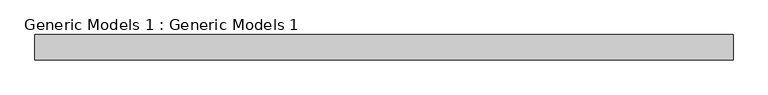
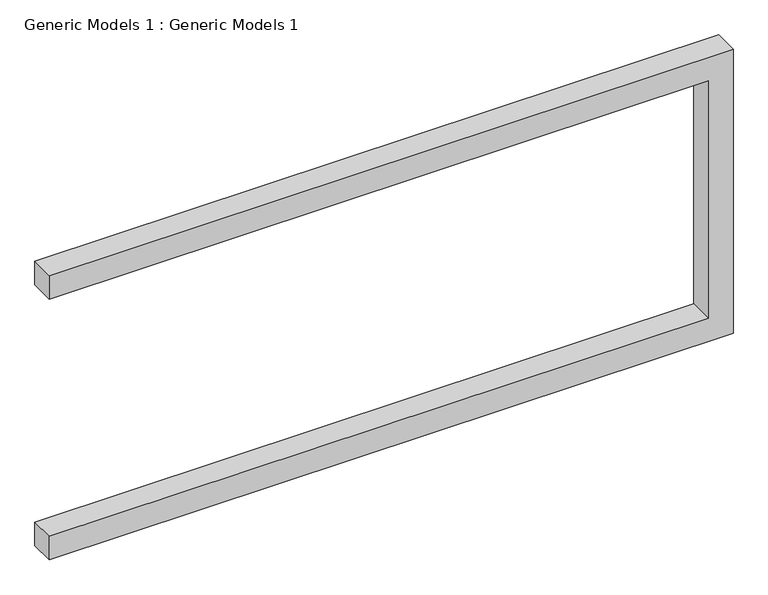
"""IFC4 building model written with IfcOpenShell, lengths in millimetres: proxy geometry, Generic Models 1 : Generic Models 1."""

from ifc_helpers import new_model, si_unit, frame, origin, place, context, project, spatial, polyline, outline, extrude, source, transform, mapped, element, save


def generic_models_1_generic_models_1_e2d67b9d(model_context):
    return source(origin(), model_context, "Body", "SweptSolid", [
        extrude(outline(polyline([(6400.8, -13179.0672301), (6096.0, -13179.0672301), (6096.0, -5101.8672301), (3022.6, -5101.8672301), (3022.6, -13179.0672301), (2717.8, -13179.0672301), (2717.8, -4797.0672301), (6400.8, -4797.0672301), (6400.8, -13179.0672301)])), frame((0.0, -7570.0302427, 0.0), z_axis=(0.0, 1.0, 0.0), x_axis=(0.0, 0.0, 1.0)), (0.0, 0.0, 1.0), 304.8),
    ])


if __name__ == "__main__":
    model = new_model("IFC4")
    model_context = context("Model", 3, world=origin())
    ifc_project = project(units=[si_unit("LENGTHUNIT", "METRE", prefix="MILLI")], contexts=[model_context])
    site = spatial("IfcSite", under=ifc_project)
    building = spatial("IfcBuilding", under=site)
    placement = place(None, origin())
    generic_models_1_generic_models_1_shape = generic_models_1_generic_models_1_e2d67b9d(model_context)
    element("IfcBuildingElementProxy", 1, Name="Generic Models 1 : Generic Models 1", ObjectType="Generic Models 1 : Generic Models 1", at=placement, inside=building, context=model_context, shape_type="MappedRepresentation", body=[
        mapped(generic_models_1_generic_models_1_shape, transform((0.0, 0.0, 0.0), x_axis=(1.0, 0.0, 0.0), y_axis=(0.0, 1.0, 0.0), z_axis=(0.0, 0.0, 1.0))),
    ])
    save(model, "model.ifc")

# Revit data of these elements
# Element 1 (IfcBuildingElementProxy, "Generic Models 1 : Generic Models 1")
#   Materials on its faces: "MARBLE FLOORING 6\""
# Materials
#   "MARBLE FLOORING 6\"": class "Generic", colour RGB 120 120 120, transparency 0, Cost = 0
